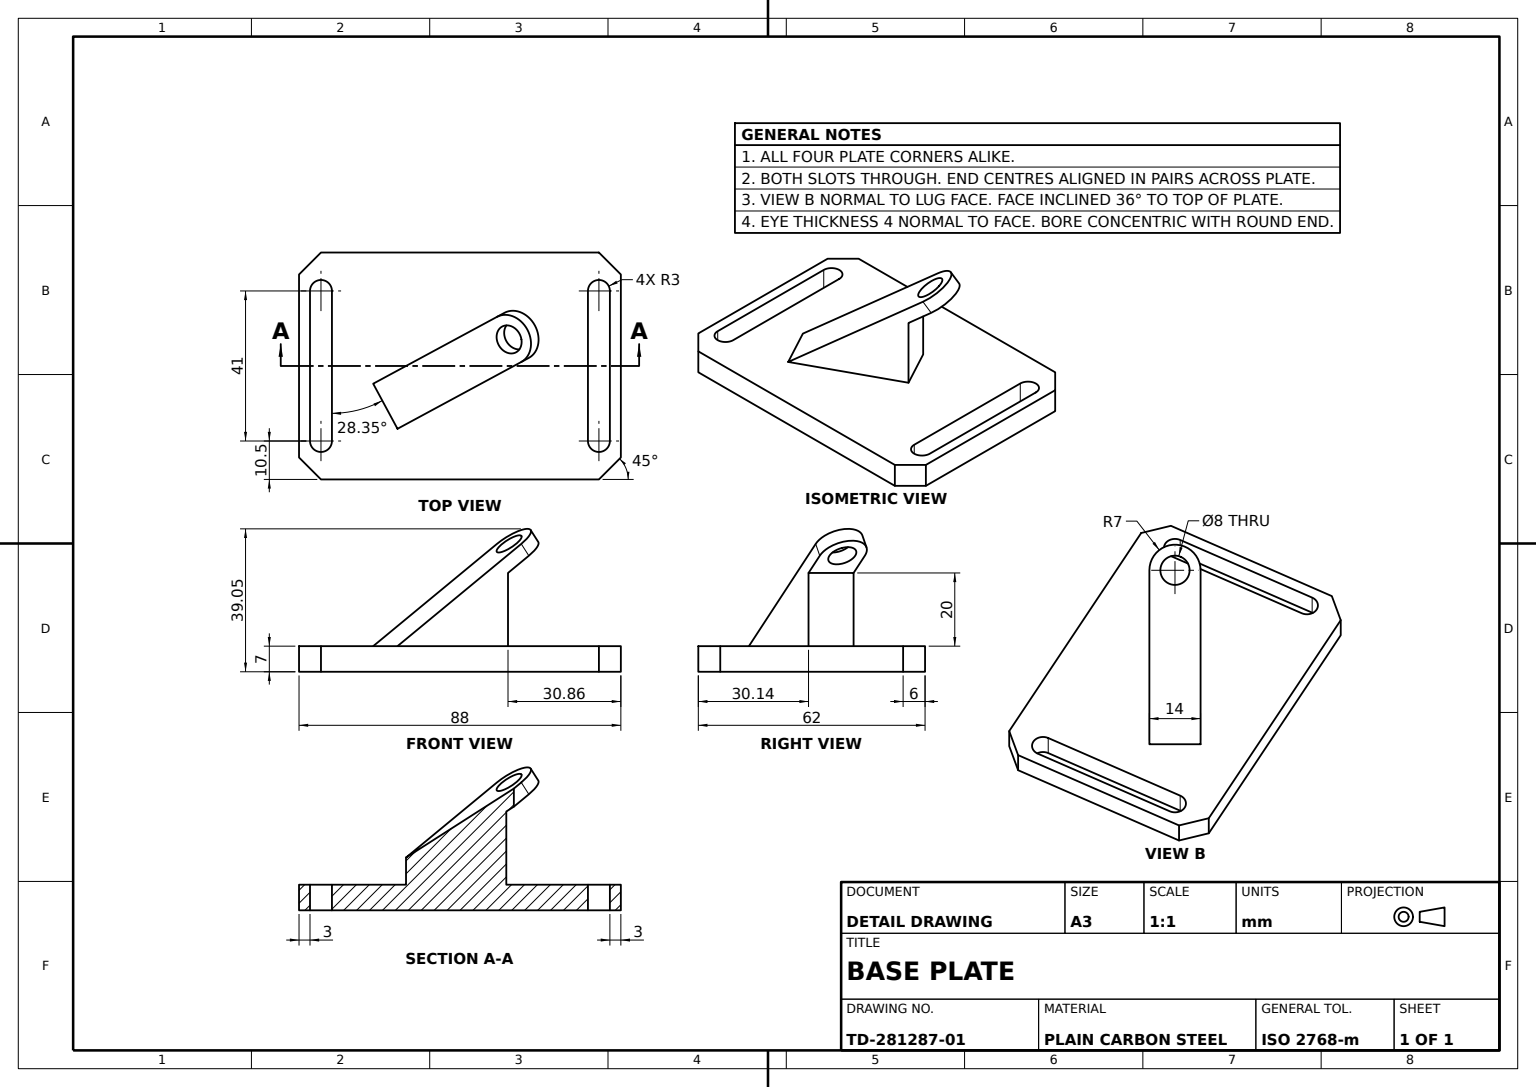
SolidWorks part; units mm, degrees
material "Plain Carbon Steel"
ref_plane "Front Plane" through (0, 0, 0) normal (0, 0, 1) x (1, 0, 0)
ref_plane "Top Plane" through (0, 0, 0) normal (0, 1, 0) x (1, 0, 0)
ref_plane "Right Plane" through (0, 0, 0) normal (1, 0, 0) x (0, 0, -1)
sketch "Base Plate Sketch" plane through (0, 0, 0) normal (0, 1, 0) x (1, 0, 0)
  line L0 (-44, 25) -> (-38, 31)
  line L1 (-38, 31) -> (38, 31)
  line L2 (-44, 25) -> (-44, -25)
  line L3 (-38, -31) -> (38, -31)
  line L4 (44, 25) -> (44, -25)
  line L5 (-44, 31) -> (44, -31) construction
  line L6 (-44, -31) -> (44, 31) construction
  line L7 (-44, -25) -> (-38, -31)
  line L8 (38, -31) -> (44, -25)
  line L9 (38, 31) -> (44, 25)
  line L10 (-38, -20.5) -> (-38, 20.5) construction
  line L11 (-41, -20.5) -> (-41, 20.5)
  line L12 (-35, -20.5) -> (-35, 20.5)
  line L13 (0, 0) -> (0, 35.9755) construction
  line L14 (38, -20.5) -> (38, 20.5) construction
  line L15 (41, -20.5) -> (41, 20.5)
  line L16 (35, -20.5) -> (35, 20.5)
  arc A0 (-41, -20.5) -> (-35, -20.5) centre (-38, -20.5) ccw
  arc A1 (-35, 20.5) -> (-41, 20.5) centre (-38, 20.5) ccw
  arc A2 (41, -20.5) -> (35, -20.5) centre (38, -20.5) cw
  arc A3 (35, 20.5) -> (41, 20.5) centre (38, 20.5) cw
  point P0 (0, 0)
  point P16 (-38, 0)
  point P25 (38, 0)
  dimension "D1" = 88
  dimension "D2" = 62
  dimension "D3" = 6
  dimension "D4" = 45
  dimension "D5" = 6
  dimension "D6" = 45
  dimension "D7" = 6
  dimension "D8" = 45
  dimension "D9" = 6
  dimension "D10" = 45
  dimension "D11" = 6
  dimension "D12" = 6
  dimension "D13" = 41
extrude "Base Plate 88x62x7" add sketch "Base Plate Sketch" along normal mid plane 7
sketch "Lug Plane Reference Sketch" plane through (0, 3.5, 0) normal (0, 1, 0) x (1, 0, 0)
  line L0 (0, 0) -> (38, 20.5) construction
  line L2 (0, 0) -> (-38, -20.5) construction
ref_plane "Lug Plane" through (0, 0, 0) normal (0.4748, 0, 0.8801) x (0.8801, 0, -0.4748)
sketch "Lug Profile Sketch" plane through (0, 0, 0) normal (0.4748, 0, 0.8801) x (0.8801, 0, -0.4748)
  line L0 (-23.177, 3.5) -> (15.2769, 31.4383)
  line L1 (0, 3.5) -> (43.177, 3.5) construction
  line L2 (11.1559, 3.5) -> (11.1559, 23.5)
  line L3 (0, 3.5) -> (-43.177, 3.5) construction
  line L4 (11.1559, 23.5) -> (17.628, 28.2023)
  line L5 (17.628, 28.2023) -> (15.2769, 31.4383)
  line L6 (-23.177, 3.5) -> (11.1559, 3.5)
  dimension "D1" = 20
  dimension "D2" = 36
  dimension "D3" = 20
  dimension "D4" = 4
  dimension "D5" = 8
extrude "Lifting Lug" add sketch "Lug Profile Sketch" along normal mid plane 14
sketch "Lug Eye Boss Sketch" plane through (-8.5121, 13.3121, 4.5921) normal (-0.5173, 0.809, 0.2791) x (0.8558, 0.489, 0.1687)
  line L0 (29.5406, 11.2849) -> (21.7735, 22.9327) construction
  circle A2 centre (25.6571, 17.1088) radius 7
extrude "Lug Eye Boss" add sketch "Lug Eye Boss Sketch" against normal blind 4
sketch "Eye Hole Sketch" plane through (-8.5121, 13.3121, 4.5921) normal (-0.5173, 0.809, 0.2791) x (0.8558, 0.489, 0.1687)
  circle A0 centre (25.6571, 17.1088) radius 4
  dimension "D1" = 8
extrude "Eye Hole Ø8" cut sketch "Eye Hole Sketch" against normal blind 4
